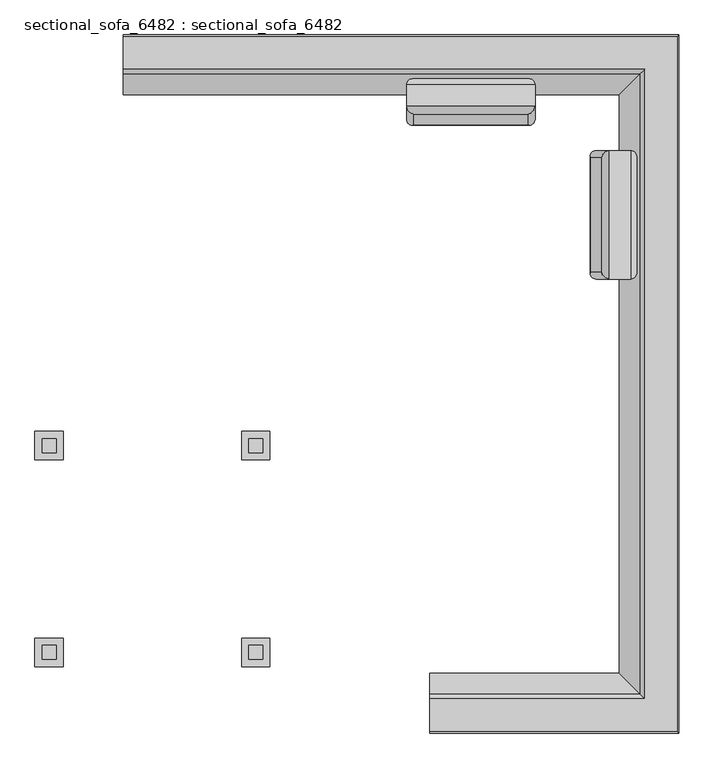
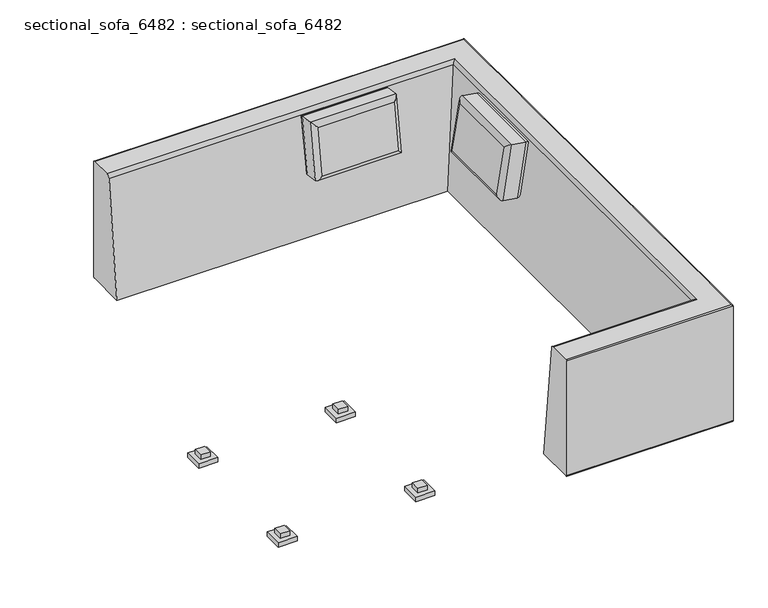
"""IFC4 building model written with IfcOpenShell, lengths in millimetres: proxy geometry, sectional_sofa_6482 : sectional_sofa_6482."""

from ifc_helpers import new_model, si_unit, frame, origin, place, context, project, spatial, circle_curve, ellipse_curve, faceted_brep, source, transform, mapped, element, save
from ifc_brep_helpers import plane_surface, cylinder_surface, advanced_brep


def sectional_sofa_6482_sectional_sofa_6482_9496661e(model_context):
    return source(origin(), model_context, "Body", "SolidModel", [
        advanced_brep(
        [(-712.932438, 1291.6931081, 704.85), (-712.932438, 1291.6931081, 57.15), (-712.932438, 1285.3431081, 50.8), (-712.932438, 1078.6460027, 50.8), (-712.932438, 1150.9219827, 695.9470238), (-712.932438, 1169.5897386, 711.2), (-712.932438, 1285.3431081, 711.2), (1268.267562, 1291.6931081, 704.85), (1268.267562, 1291.6931081, 57.15), (1261.917562, 1285.3431081, 50.8), (1261.917562, -1191.1568919, 50.8), (379.267562, -1191.1568919, 50.8), (379.267562, -984.4597865, 50.8), (1055.2204567, -984.4597865, 50.8), (1055.2204567, 1078.6460027, 50.8), (1127.4964367, 1150.9219827, 695.9470238), (1146.1641926, 1169.5897386, 711.2), (1146.1641926, -1075.4035225, 711.2), (379.267562, -1075.4035225, 711.2), (379.267562, -1191.1568919, 711.2), (1261.917562, -1191.1568919, 711.2), (1261.917562, 1285.3431081, 711.2), (1268.267562, -1197.5068919, 704.85), (1268.267562, -1197.5068919, 57.15), (1127.4964367, -1056.7357665, 695.9470238), (379.267562, -1197.5068919, 57.15), (379.267562, -1197.5068919, 704.85), (379.267562, -1056.7357665, 695.9470238)],
        [
            (0, 1),
            (1, 2, circle_curve(frame((-712.932438, 1285.3431081, 57.15), z_axis=(-1.0, 0.0, 0.0), x_axis=(0.0, -1.0, 0.0)), 6.35)),
            (2, 3),
            (3, 4, circle_curve(frame((-712.932438, 4725.645818, -31.1522279), z_axis=(-1.0, 0.0, 0.0), x_axis=(0.0, -1.0, 0.0)), 3647.9204789)),
            (4, 5, circle_curve(frame((-712.932438, 1169.5897386, 692.15), z_axis=(-1.0, 0.0, 0.0), x_axis=(0.0, -1.0, 0.0)), 19.05)),
            (5, 6),
            (6, 0, circle_curve(frame((-712.932438, 1285.3431081, 704.85), z_axis=(-1.0, 0.0, 0.0), x_axis=(0.0, -1.0, 0.0)), 6.35)),
            (0, 7),
            (7, 8),
            (8, 1),
            (8, 9, ellipse_curve(frame((1261.917562, 1285.3431081, 57.15), z_axis=(-0.7071067811865475, 0.7071067811865475, 0.0), x_axis=(-0.7071067811865476, -0.7071067811865474, 0.0)), 8.9802561, 6.35)),
            (9, 2),
            (9, 10),
            (10, 11),
            (11, 12),
            (12, 13),
            (13, 14),
            (14, 3),
            (14, 15, ellipse_curve(frame((4702.2202719, 4725.645818, -31.1522279), z_axis=(-0.7071067811865475, 0.7071067811865475, 0.0), x_axis=(-0.7071067811865476, -0.7071067811865474, 0.0)), 5158.9386157, 3647.9204789)),
            (15, 4),
            (15, 16, ellipse_curve(frame((1146.1641926, 1169.5897386, 692.15), z_axis=(-0.7071067811865475, 0.7071067811865475, 0.0), x_axis=(-0.7071067811865476, -0.7071067811865474, 0.0)), 26.9407684, 19.05)),
            (16, 5),
            (16, 17),
            (17, 18),
            (18, 19),
            (19, 20),
            (20, 21),
            (21, 6),
            (21, 7, ellipse_curve(frame((1261.917562, 1285.3431081, 704.85), z_axis=(-0.7071067811865475, 0.7071067811865475, 0.0), x_axis=(-0.7071067811865476, -0.7071067811865474, 0.0)), 8.9802561, 6.35)),
            (7, 22),
            (22, 23),
            (23, 8),
            (23, 10, ellipse_curve(frame((1261.917562, -1191.1568919, 57.15), z_axis=(0.7071067811865475, 0.7071067811865475, 0.0), x_axis=(-0.7071067811865474, 0.7071067811865476, 0.0)), 8.9802561, 6.35)),
            (13, 24, ellipse_curve(frame((4702.2202719, -4631.4596018, -31.1522279), z_axis=(0.7071067811865475, 0.7071067811865475, 0.0), x_axis=(-0.7071067811865474, 0.7071067811865476, 0.0)), 5158.9386157, 3647.9204789)),
            (24, 15),
            (24, 17, ellipse_curve(frame((1146.1641926, -1075.4035225, 692.15), z_axis=(0.7071067811865475, 0.7071067811865475, 0.0), x_axis=(-0.7071067811865474, 0.7071067811865476, 0.0)), 26.9407684, 19.05)),
            (20, 22, ellipse_curve(frame((1261.917562, -1191.1568919, 704.85), z_axis=(0.7071067811865475, 0.7071067811865475, 0.0), x_axis=(-0.7071067811865474, 0.7071067811865476, 0.0)), 8.9802561, 6.35)),
            (11, 25, circle_curve(frame((379.267562, -1191.1568919, 57.15), z_axis=(-1.0, 0.0, 0.0), x_axis=(0.0, 1.0, 0.0)), 6.35)),
            (25, 26),
            (26, 19, circle_curve(frame((379.267562, -1191.1568919, 704.85), z_axis=(-1.0, 0.0, 0.0), x_axis=(0.0, 1.0, 0.0)), 6.35)),
            (18, 27, circle_curve(frame((379.267562, -1075.4035225, 692.15), z_axis=(-1.0, 0.0, 0.0), x_axis=(0.0, 1.0, 0.0)), 19.05)),
            (27, 12, circle_curve(frame((379.267562, -4631.4596018, -31.1522279), z_axis=(-1.0, 0.0, 0.0), x_axis=(0.0, 1.0, 0.0)), 3647.9204789)),
            (22, 26),
            (25, 23),
            (27, 24),
        ],
        [
            plane_surface(frame((-712.932438, 1291.6931081, 50.8), z_axis=(-1.0, 0.0, 0.0), x_axis=(0.0, 0.0, -1.0))),
            plane_surface(frame((-712.932438, 1291.6931081, 704.85), z_axis=(0.0, 1.0, 0.0), x_axis=(1.0, 0.0, 0.0))),
            cylinder_surface(frame((-712.932438, 1285.3431081, 57.15), z_axis=(-1.0, 0.0, 0.0), x_axis=(0.0, -1.0, 0.0)), 6.35),
            plane_surface(frame((-712.932438, 1285.3431081, 50.8), z_axis=(0.0, 0.0, -1.0), x_axis=(1.0, 0.0, 0.0))),
            cylinder_surface(frame((-712.932438, 4725.645818, -31.1522279), z_axis=(-1.0, 0.0, 0.0), x_axis=(0.0, -1.0, 0.0)), 3647.9204789),
            cylinder_surface(frame((-712.932438, 1169.5897386, 692.15), z_axis=(-1.0, 0.0, 0.0), x_axis=(0.0, -1.0, 0.0)), 19.05),
            plane_surface(frame((-712.932438, 1169.5897386, 711.2), z_axis=(0.0, 0.0, 1.0), x_axis=(1.0, 0.0, 0.0))),
            cylinder_surface(frame((-712.932438, 1285.3431081, 704.85), z_axis=(-1.0, 0.0, 0.0), x_axis=(0.0, -1.0, 0.0)), 6.35),
            plane_surface(frame((1268.267562, 1291.6931081, 704.85), z_axis=(1.0, 0.0, 0.0), x_axis=(0.0, -1.0, 0.0))),
            cylinder_surface(frame((1261.917562, 1291.6931081, 57.15), z_axis=(0.0, 1.0, 0.0), x_axis=(-1.0, 0.0, 0.0)), 6.35),
            cylinder_surface(frame((4702.2202719, 1291.6931081, -31.1522279), z_axis=(0.0, 1.0, 0.0), x_axis=(-1.0, 0.0, 0.0)), 3647.9204789),
            cylinder_surface(frame((1146.1641926, 1291.6931081, 692.15), z_axis=(0.0, 1.0, 0.0), x_axis=(-1.0, 0.0, 0.0)), 19.05),
            cylinder_surface(frame((1261.917562, 1291.6931081, 704.85), z_axis=(0.0, 1.0, 0.0), x_axis=(-1.0, 0.0, 0.0)), 6.35),
            plane_surface(frame((379.267562, -1197.5068919, 50.8), z_axis=(-1.0, 0.0, 0.0), x_axis=(0.0, 0.0, -1.0))),
            plane_surface(frame((1268.267562, -1197.5068919, 704.85), z_axis=(0.0, -1.0, 0.0), x_axis=(-1.0, 0.0, 0.0))),
            cylinder_surface(frame((1268.267562, -1191.1568919, 57.15), z_axis=(1.0, 0.0, 0.0), x_axis=(0.0, 1.0, 0.0)), 6.35),
            cylinder_surface(frame((1268.267562, -4631.4596018, -31.1522279), z_axis=(1.0, 0.0, 0.0), x_axis=(0.0, 1.0, 0.0)), 3647.9204789),
            cylinder_surface(frame((1268.267562, -1075.4035225, 692.15), z_axis=(1.0, 0.0, 0.0), x_axis=(0.0, 1.0, 0.0)), 19.05),
            cylinder_surface(frame((1268.267562, -1191.1568919, 704.85), z_axis=(1.0, 0.0, 0.0), x_axis=(0.0, 1.0, 0.0)), 6.35),
        ],
        [
            (0, [[1, 2, 3, 4, 5, 6, 7]]),
            (1, [[-1, 8, 9, 10]]),
            (2, [[-2, -10, 11, 12]]),
            (3, [[-3, -12, 13, 14, 15, 16, 17, 18]]),
            (4, [[-4, -18, 19, 20]]),
            (5, [[-5, -20, 21, 22]]),
            (6, [[-6, -22, 23, 24, 25, 26, 27, 28]]),
            (7, [[-7, -28, 29, -8]]),
            (8, [[-9, 30, 31, 32]]),
            (9, [[-11, -32, 33, -13]]),
            (10, [[-17, 34, 35, -19]]),
            (11, [[-21, -35, 36, -23]]),
            (12, [[-27, 37, -30, -29]]),
            (13, [[-15, 38, 39, 40, -25, 41, 42]]),
            (14, [[-31, 43, -39, 44]]),
            (15, [[-14, -33, -44, -38]]),
            (16, [[-16, -42, 45, -34]]),
            (17, [[-24, -36, -45, -41]]),
            (18, [[-26, -40, -43, -37]]),
        ],
    ),
        advanced_brep(
        [(754.9501866, 990.6789418, 428.302718), (754.9501866, 1065.9407934, 416.3824117), (754.9501866, 1113.6220183, 717.429818), (754.9501866, 1038.3601668, 729.3501242), (297.7501866, 1038.3601668, 729.3501242), (297.7501866, 1113.6220183, 717.429818), (297.7501866, 1065.9407934, 416.3824117), (297.7501866, 990.6789418, 428.302718), (323.1501866, 1095.0015126, 437.4962602), (323.1501866, 1134.7358668, 688.3690987), (729.5501866, 1134.7358668, 688.3690987), (729.5501866, 1095.0015126, 437.4962602), (323.1501866, 1009.2994475, 708.2362758), (323.1501866, 969.5650934, 457.3634372), (729.5501866, 969.5650934, 457.3634372), (729.5501866, 1009.2994475, 708.2362758)],
        [
            (0, 1),
            (1, 2),
            (2, 3),
            (3, 0),
            (4, 5),
            (5, 6),
            (6, 7),
            (7, 4),
            (0, 7),
            (6, 1),
            (8, 9),
            (9, 10),
            (10, 11),
            (11, 8),
            (2, 5),
            (4, 3),
            (12, 13),
            (13, 14),
            (14, 15),
            (15, 12),
            (7, 13, ellipse_curve(frame((323.1501866, 994.6523772, 453.3900018), z_axis=(-0.7071067811865474, 0.1106158710412283, 0.6984011233337117), x_axis=(-0.7071067811865474, -0.11061587104122816, -0.6984011233337117)), 35.9210245, 25.4)),
            (12, 4, ellipse_curve(frame((323.1501866, 1034.3867314, 704.2628403), z_axis=(-0.7071067811865476, -0.11061587104122826, -0.6984011233337116), x_axis=(0.7071067811865475, -0.11061587104122819, -0.6984011233337117)), 35.9210245, 25.4)),
            (8, 6, ellipse_curve(frame((323.1501866, 1069.9142288, 441.4696956), z_axis=(-0.7071067811865474, 0.11061587104122826, 0.6984011233337117), x_axis=(-0.7071067811865474, -0.11061587104122816, -0.6984011233337117)), 35.9210245, 25.4)),
            (5, 9, ellipse_curve(frame((323.1501866, 1109.6485829, 692.3425341), z_axis=(-0.7071067811865476, -0.11061587104122823, -0.6984011233337116), x_axis=(0.7071067811865475, -0.11061587104122819, -0.6984011233337117)), 35.9210245, 25.4)),
            (0, 14, ellipse_curve(frame((729.5501866, 994.6523772, 453.3900018), z_axis=(-0.7071067811865476, -0.11061587104122807, -0.6984011233337117), x_axis=(0.7071067811865475, -0.11061587104122819, -0.6984011233337117)), 35.9210245, 25.4)),
            (11, 1, ellipse_curve(frame((729.5501866, 1069.9142288, 441.4696956), z_axis=(-0.7071067811865476, -0.11061587104122811, -0.6984011233337117), x_axis=(0.7071067811865475, -0.11061587104122819, -0.6984011233337117)), 35.9210245, 25.4)),
            (3, 15, ellipse_curve(frame((729.5501866, 1034.3867314, 704.2628403), z_axis=(0.7071067811865475, -0.1106158710412281, -0.6984011233337117), x_axis=(0.7071067811865474, 0.11061587104122819, 0.6984011233337117)), 35.9210245, 25.4)),
            (10, 2, ellipse_curve(frame((729.5501866, 1109.6485829, 692.3425341), z_axis=(0.7071067811865474, -0.11061587104122812, -0.6984011233337117), x_axis=(0.7071067811865475, 0.1106158710412282, 0.6984011233337118)), 35.9210245, 25.4)),
        ],
        [
            plane_surface(frame((754.9501866, 1077.8583572, 254.0), z_axis=(1.0, 0.0, 0.0), x_axis=(0.0, 0.0, 1.0))),
            plane_surface(frame((297.7501866, 1077.8583572, 254.0), z_axis=(-1.0, 0.0, 0.0), x_axis=(0.0, 0.0, 1.0))),
            plane_surface(frame((754.9501866, 965.591658, 432.2761534), z_axis=(0.0, -0.15643446504021818, -0.9876883405951399), x_axis=(-1.0, 0.0, 0.0))),
            plane_surface(frame((754.9501866, 1091.0280772, 412.4089763), z_axis=(0.0, 0.9876883405951399, -0.15643446504021818), x_axis=(-1.0, 0.0, 0.0))),
            plane_surface(frame((754.9501866, 1138.7093022, 713.4563825), z_axis=(0.0, 0.15643446504021818, 0.9876883405951399), x_axis=(-1.0, 0.0, 0.0))),
            plane_surface(frame((754.9501866, 1013.2728829, 733.3235596), z_axis=(0.0, -0.9876883405951399, 0.15643446504021818), x_axis=(-1.0, 0.0, 0.0))),
            cylinder_surface(frame((323.1501866, 1038.3601668, 729.3501242), z_axis=(0.0, -0.15643446504021827, -0.9876883405951398), x_axis=(1.0, 0.0, 0.0)), 25.4),
            cylinder_surface(frame((323.1501866, 1113.6220183, 717.429818), z_axis=(0.0, -0.15643446504021824, -0.9876883405951398), x_axis=(1.0, 0.0, 0.0)), 25.4),
            cylinder_surface(frame((297.7501866, 994.6523772, 453.3900018), z_axis=(1.0, 0.0, 0.0), x_axis=(0.0, 0.15643446504021824, 0.9876883405951398)), 25.4),
            cylinder_surface(frame((297.7501866, 1069.9142288, 441.4696956), z_axis=(1.0, 0.0, 0.0), x_axis=(0.0, 0.15643446504021957, 0.9876883405951395)), 25.4),
            cylinder_surface(frame((729.5501866, 990.6789418, 428.302718), z_axis=(0.0, 0.15643446504021813, 0.9876883405951398), x_axis=(-1.0, 0.0, 0.0)), 25.4),
            cylinder_surface(frame((729.5501866, 1065.9407934, 416.3824117), z_axis=(0.0, 0.15643446504021816, 0.9876883405951398), x_axis=(-1.0, 0.0, 0.0)), 25.4),
            cylinder_surface(frame((754.9501866, 1034.3867314, 704.2628403), z_axis=(-1.0, 0.0, 0.0), x_axis=(0.0, -0.15643446504021813, -0.9876883405951398)), 25.4),
            cylinder_surface(frame((754.9501866, 1109.6485829, 692.3425341), z_axis=(-1.0, 0.0, 0.0), x_axis=(0.0, -0.1564344650402168, -0.98768834059514)), 25.4),
        ],
        [
            (0, [[1, 2, 3, 4]]),
            (1, [[5, 6, 7, 8]]),
            (2, [[-1, 9, -7, 10]]),
            (3, [[11, 12, 13, 14]]),
            (4, [[-3, 15, -5, 16]]),
            (5, [[17, 18, 19, 20]]),
            (6, [[21, -17, 22, -8]]),
            (7, [[23, -6, 24, -11]]),
            (8, [[-21, -9, 25, -18]]),
            (9, [[-23, -14, 26, -10]]),
            (10, [[-25, -4, 27, -19]]),
            (11, [[-26, -13, 28, -2]]),
            (12, [[-22, -20, -27, -16]]),
            (13, [[-24, -15, -28, -12]]),
        ],
    ),
        advanced_brep(
        [(972.5408994, 421.3757369, 422.7530414), (1047.802751, 421.3757369, 410.8327352), (1095.4839759, 421.3757369, 711.8801414), (1020.2221244, 421.3757369, 723.8004476), (1020.2221244, 878.5757369, 723.8004476), (1095.4839759, 878.5757369, 711.8801414), (1047.802751, 878.5757369, 410.8327352), (972.5408994, 878.5757369, 422.7530414), (1076.8634702, 853.1757369, 431.9465836), (1116.5978244, 853.1757369, 682.8194221), (1116.5978244, 446.7757369, 682.8194221), (1076.8634702, 446.7757369, 431.9465836), (991.1614051, 853.1757369, 702.6865992), (951.427051, 853.1757369, 451.8137607), (951.427051, 446.7757369, 451.8137607), (991.1614051, 446.7757369, 702.6865992)],
        [
            (0, 1),
            (1, 2),
            (2, 3),
            (3, 0),
            (4, 5),
            (5, 6),
            (6, 7),
            (7, 4),
            (0, 7),
            (6, 1),
            (8, 9),
            (9, 10),
            (10, 11),
            (11, 8),
            (2, 5),
            (4, 3),
            (12, 13),
            (13, 14),
            (14, 15),
            (15, 12),
            (7, 13, ellipse_curve(frame((976.5143348, 853.1757369, 447.8403253), z_axis=(0.11061587104122693, 0.7071067811865475, 0.698401123333712), x_axis=(-0.11061587104122939, 0.7071067811865475, -0.6984011233337115)), 35.9210245, 25.4)),
            (12, 4, ellipse_curve(frame((1016.248689, 853.1757369, 698.7131638), z_axis=(-0.11061587104122933, 0.7071067811865474, -0.6984011233337116), x_axis=(-0.11061587104122698, -0.7071067811865476, -0.6984011233337118)), 35.9210245, 25.4)),
            (8, 6, ellipse_curve(frame((1051.7761864, 853.1757369, 435.920019), z_axis=(0.11061587104122693, 0.7071067811865475, 0.698401123333712), x_axis=(-0.11061587104122939, 0.7071067811865475, -0.6984011233337115)), 35.9210245, 25.4)),
            (5, 9, ellipse_curve(frame((1091.5105405, 853.1757369, 686.7928575), z_axis=(-0.11061587104122934, 0.7071067811865474, -0.6984011233337116), x_axis=(-0.11061587104122697, -0.7071067811865476, -0.6984011233337118)), 35.9210245, 25.4)),
            (0, 14, ellipse_curve(frame((976.5143348, 446.7757369, 447.8403253), z_axis=(-0.11061587104122948, 0.7071067811865474, -0.6984011233337116), x_axis=(-0.11061587104122696, -0.7071067811865478, -0.6984011233337116)), 35.9210245, 25.4)),
            (11, 1, ellipse_curve(frame((1051.7761864, 446.7757369, 435.920019), z_axis=(-0.11061587104122947, 0.7071067811865474, -0.6984011233337116), x_axis=(-0.11061587104122693, -0.7071067811865478, -0.6984011233337116)), 35.9210245, 25.4)),
            (3, 15, ellipse_curve(frame((1016.248689, 446.7757369, 698.7131638), z_axis=(-0.11061587104122703, -0.7071067811865477, -0.6984011233337116), x_axis=(0.11061587104122943, -0.7071067811865472, 0.6984011233337117)), 35.9210245, 25.4)),
            (10, 2, ellipse_curve(frame((1091.5105405, 446.7757369, 686.7928575), z_axis=(-0.11061587104122698, -0.7071067811865477, -0.6984011233337116), x_axis=(0.11061587104122943, -0.7071067811865472, 0.6984011233337117)), 35.9210245, 25.4)),
        ],
        [
            plane_surface(frame((1059.7203148, 421.3757369, 248.4503234), z_axis=(0.0, -1.0, 0.0), x_axis=(0.0, 0.0, 1.0))),
            plane_surface(frame((1059.7203148, 878.5757369, 248.4503234), z_axis=(0.0, 1.0, 0.0), x_axis=(0.0, 0.0, 1.0))),
            plane_surface(frame((947.4536156, 421.3757369, 426.7264768), z_axis=(-0.15643446504021818, 0.0, -0.9876883405951399), x_axis=(0.0, 1.0, 0.0))),
            plane_surface(frame((1072.8900348, 421.3757369, 406.8592998), z_axis=(0.9876883405951399, 0.0, -0.15643446504021818), x_axis=(0.0, 1.0, 0.0))),
            plane_surface(frame((1120.5712598, 421.3757369, 707.906706), z_axis=(0.15643446504021818, 0.0, 0.9876883405951399), x_axis=(0.0, 1.0, 0.0))),
            plane_surface(frame((995.1348405, 421.3757369, 727.773883), z_axis=(-0.9876883405951399, 0.0, 0.15643446504021818), x_axis=(0.0, 1.0, 0.0))),
            cylinder_surface(frame((1020.2221244, 853.1757369, 723.8004476), z_axis=(-0.15643446504021816, 0.0, -0.9876883405951398), x_axis=(0.0, -1.0, 0.0)), 25.4),
            cylinder_surface(frame((1095.4839759, 853.1757369, 711.8801414), z_axis=(-0.15643446504021816, 0.0, -0.9876883405951398), x_axis=(0.0, -1.0, 0.0)), 25.4),
            cylinder_surface(frame((976.5143348, 878.5757369, 447.8403253), z_axis=(0.0, -1.0000000000000002, 0.0), x_axis=(0.15643446504021824, 0.0, 0.9876883405951399)), 25.4),
            cylinder_surface(frame((1051.7761864, 878.5757369, 435.920019), z_axis=(0.0, -1.0000000000000002, 0.0), x_axis=(0.15643446504022113, 0.0, 0.9876883405951394)), 25.4),
            cylinder_surface(frame((972.5408994, 446.7757369, 422.7530414), z_axis=(0.15643446504021827, 0.0, 0.9876883405951398), x_axis=(0.0, 1.0, 0.0)), 25.4),
            cylinder_surface(frame((1047.802751, 446.7757369, 410.8327352), z_axis=(0.15643446504021824, 0.0, 0.9876883405951398), x_axis=(0.0, 1.0, 0.0)), 25.4),
            cylinder_surface(frame((1016.248689, 421.3757369, 698.7131638), z_axis=(0.0, 1.0000000000000002, 0.0), x_axis=(-0.15643446504021816, 0.0, -0.9876883405951399)), 25.4),
            cylinder_surface(frame((1091.5105405, 421.3757369, 686.7928575), z_axis=(0.0, 1.0000000000000002, 0.0), x_axis=(-0.1564344650402153, 0.0, -0.9876883405951403)), 25.4),
        ],
        [
            (0, [[1, 2, 3, 4]]),
            (1, [[5, 6, 7, 8]]),
            (2, [[-1, 9, -7, 10]]),
            (3, [[11, 12, 13, 14]]),
            (4, [[-3, 15, -5, 16]]),
            (5, [[17, 18, 19, 20]]),
            (6, [[21, -17, 22, -8]]),
            (7, [[23, -6, 24, -11]]),
            (8, [[-21, -9, 25, -18]]),
            (9, [[-23, -14, 26, -10]]),
            (10, [[-25, -4, 27, -19]]),
            (11, [[-26, -13, 28, -2]]),
            (12, [[-22, -20, -27, -16]]),
            (13, [[-24, -15, -28, -12]]),
        ],
    ),
        faceted_brep([(-926.5924005, -223.6520518, 25.4), (-926.5924005, -122.0520518, 25.4), (-1028.1924005, -122.0520518, 25.4), (-1028.1924005, -223.6520518, 25.4), (-951.9924005, -147.4520518, 25.4), (-951.9924005, -198.2520518, 25.4), (-1002.7924005, -198.2520518, 25.4), (-1002.7924005, -147.4520518, 25.4), (-926.5924005, -223.6520518, 0.0), (-1028.1924005, -223.6520518, 0.0), (-1028.1924005, -122.0520518, 0.0), (-926.5924005, -122.0520518, 0.0), (-951.9924005, -198.2520518, 50.8), (-951.9924005, -147.4520518, 50.8), (-1002.7924005, -147.4520518, 50.8), (-1002.7924005, -198.2520518, 50.8)], [[[0, 1, 2, 3], [4, 5, 6, 7]], [[8, 9, 10, 11]], [[1, 0, 8, 11]], [[2, 1, 11, 10]], [[3, 2, 10, 9]], [[0, 3, 9, 8]], [[12, 13, 14, 15]], [[13, 12, 5, 4]], [[14, 13, 4, 7]], [[15, 14, 7, 6]], [[12, 15, 6, 5]]]),
        faceted_brep([(-291.5924005, -223.6520518, 25.4), (-189.9924005, -223.6520518, 25.4), (-189.9924005, -122.0520518, 25.4), (-291.5924005, -122.0520518, 25.4), (-215.3924005, -198.2520518, 25.4), (-266.1924005, -198.2520518, 25.4), (-266.1924005, -147.4520518, 25.4), (-215.3924005, -147.4520518, 25.4), (-291.5924005, -223.6520518, 0.0), (-291.5924005, -122.0520518, 0.0), (-189.9924005, -122.0520518, 0.0), (-189.9924005, -223.6520518, 0.0), (-266.1924005, -198.2520518, 50.8), (-215.3924005, -198.2520518, 50.8), (-215.3924005, -147.4520518, 50.8), (-266.1924005, -147.4520518, 50.8)], [[[0, 1, 2, 3], [4, 5, 6, 7]], [[8, 9, 10, 11]], [[1, 0, 8, 11]], [[2, 1, 11, 10]], [[3, 2, 10, 9]], [[0, 3, 9, 8]], [[12, 13, 14, 15]], [[13, 12, 5, 4]], [[14, 13, 4, 7]], [[15, 14, 7, 6]], [[12, 15, 6, 5]]]),
        faceted_brep([(-291.5924005, -960.2520518, 25.4), (-189.9924005, -960.2520518, 25.4), (-189.9924005, -858.6520518, 25.4), (-291.5924005, -858.6520518, 25.4), (-215.3924005, -934.8520518, 25.4), (-266.1924005, -934.8520518, 25.4), (-266.1924005, -884.0520518, 25.4), (-215.3924005, -884.0520518, 25.4), (-291.5924005, -960.2520518, 0.0), (-291.5924005, -858.6520518, 0.0), (-189.9924005, -858.6520518, 0.0), (-189.9924005, -960.2520518, 0.0), (-266.1924005, -934.8520518, 50.8), (-215.3924005, -934.8520518, 50.8), (-215.3924005, -884.0520518, 50.8), (-266.1924005, -884.0520518, 50.8)], [[[0, 1, 2, 3], [4, 5, 6, 7]], [[8, 9, 10, 11]], [[1, 0, 8, 11]], [[2, 1, 11, 10]], [[3, 2, 10, 9]], [[0, 3, 9, 8]], [[12, 13, 14, 15]], [[13, 12, 5, 4]], [[14, 13, 4, 7]], [[15, 14, 7, 6]], [[12, 15, 6, 5]]]),
        faceted_brep([(-926.5924005, -960.2520518, 25.4), (-926.5924005, -858.6520518, 25.4), (-1028.1924005, -858.6520518, 25.4), (-1028.1924005, -960.2520518, 25.4), (-951.9924005, -884.0520518, 25.4), (-951.9924005, -934.8520518, 25.4), (-1002.7924005, -934.8520518, 25.4), (-1002.7924005, -884.0520518, 25.4), (-926.5924005, -960.2520518, 0.0), (-1028.1924005, -960.2520518, 0.0), (-1028.1924005, -858.6520518, 0.0), (-926.5924005, -858.6520518, 0.0), (-951.9924005, -934.8520518, 50.8), (-951.9924005, -884.0520518, 50.8), (-1002.7924005, -884.0520518, 50.8), (-1002.7924005, -934.8520518, 50.8)], [[[0, 1, 2, 3], [4, 5, 6, 7]], [[8, 9, 10, 11]], [[1, 0, 8, 11]], [[2, 1, 11, 10]], [[3, 2, 10, 9]], [[0, 3, 9, 8]], [[12, 13, 14, 15]], [[13, 12, 5, 4]], [[14, 13, 4, 7]], [[15, 14, 7, 6]], [[12, 15, 6, 5]]]),
    ])


if __name__ == "__main__":
    model = new_model("IFC4")
    model_context = context("Model", 3, world=origin())
    ifc_project = project(units=[si_unit("LENGTHUNIT", "METRE", prefix="MILLI")], contexts=[model_context])
    site = spatial("IfcSite", under=ifc_project)
    building = spatial("IfcBuilding", under=site)
    placement = place(None, origin())
    sectional_sofa_6482_sectional_sofa_6482_shape = sectional_sofa_6482_sectional_sofa_6482_9496661e(model_context)
    element("IfcBuildingElementProxy", 1, Name="sectional_sofa_6482 : sectional_sofa_6482", ObjectType="sectional_sofa_6482 : sectional_sofa_6482", at=placement, inside=building, context=model_context, shape_type="MappedRepresentation", body=[
        mapped(sectional_sofa_6482_sectional_sofa_6482_shape, transform((0.0, 0.0, 0.0), x_axis=(1.0, 0.0, 0.0), y_axis=(0.0, 1.0, 0.0), z_axis=(0.0, 0.0, 1.0))),
    ])
    save(model, "model.ifc")

# Revit data of these elements
# Type "sectional_sofa_6482 : sectional_sofa_6482"
#   frame trim = frame trim
#   fabric = Fabric
#   Frame = frame
#   FABRIC 2 = fabric 2
#   Default Elevation = 0
# Element 1 (IfcBuildingElementProxy, "sectional_sofa_6482 : sectional_sofa_6482")
#   Materials on its faces: "frame trim", "Fabric", "fabric 2", "frame"
# Materials
#   "frame trim": class "Metal", colour RGB 182 182 182, transparency 0
#   "Fabric": class "Textile", colour RGB 120 120 120, transparency 0, Description = "Fabric, gray stripes", Cost = 0
#   "frame": class "Wood", colour RGB 71 38 7, transparency 0
#   "fabric 2": class "Fabric", colour RGB 128 0 0, transparency 0
